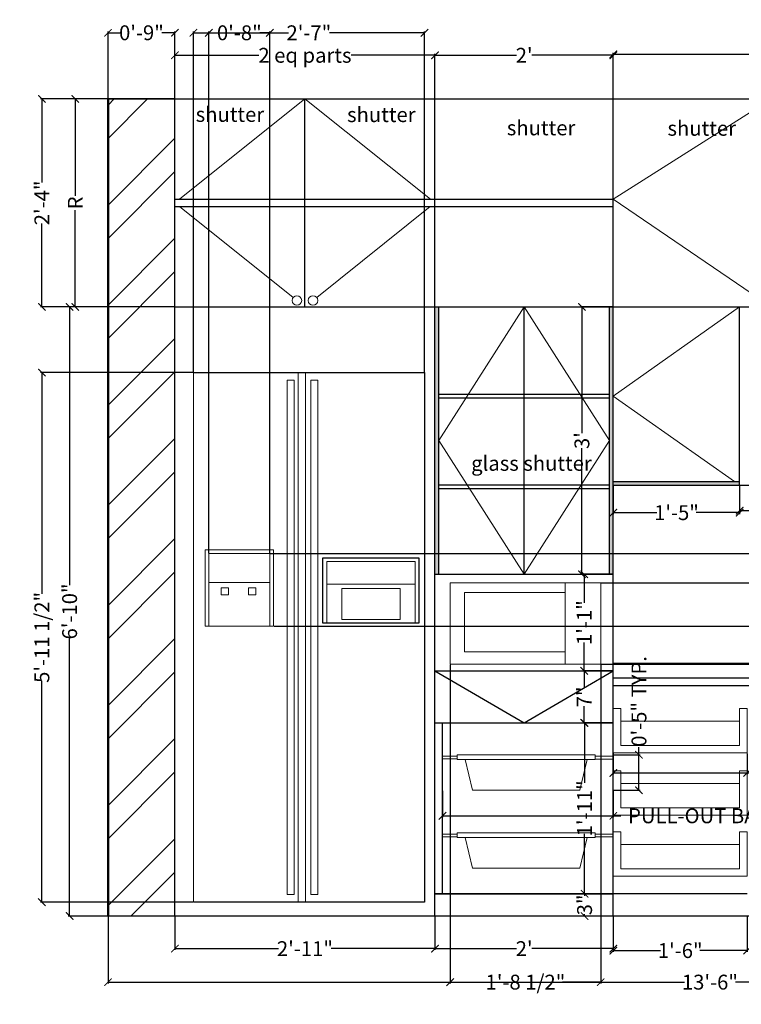
# Model space of a CAD drawing. Units: inches. Extents: x 3107 to 3291, y 1339 to 1621.
# Tile 2 of 3: x 3107 to 3204, y 1489 to 1621. Entities that reach past the tile are written whole.
import ezdxf

# ---------------------------------------------------------------- set-up
doc = ezdxf.new("R2010")
doc.units = ezdxf.units.IN
for name, color, linetype, lineweight in [('A-ANNO-DIMS', 2, 'Continuous', 18), ('A-ANNO-TEXT', 7, 'Continuous', 18), ('A-ELEV', 7, 'Continuous', 25), ('A-ELEV-OPEN', 165, 'Continuous', 13), ('A-ELEV-PATT', 8, 'Continuous', 13), ('A-EQPM', 3, 'Continuous', 18), ('A-FURN', 5, 'Continuous', 18), ('A-WALL', 7, 'Continuous', 50), ('A-WALL-PATT', 8, 'Continuous', 13)]:
    doc.layers.add(name, color=color, linetype=linetype, lineweight=lineweight)
doc.styles.get("Standard").update_dxf_attribs({"font": 'arial.ttf', "height": 2})
doc.dimstyles.get("Standard").update_dxf_attribs({"dimtxt": 2, "dimasz": 1, "dimexe": 0.18, "dimexo": 0.0625, "dimgap": 0.09, "dimtad": 0, "dimdec": 0, "dimzin": 0, "dimdsep": 46, "dimlunit": 3, "dimtxsty": 'Standard', "dimblk": 'ARCHTICK', "dimcen": 0.09, "dimadec": 0, "dimazin": 0, "dimtfac": 1, "dimtdec": 0, "dimtofl": 0, "dimtmove": 0, "dimatfit": 3, "dimfxl": 1, "dimtolj": 1, "dimtzin": 0, "dimarcsym": 0})

# ---------------------------------------------------------------- blocks, each defined once
blk = doc.blocks.new('_ArchTick')
at = {"color": 0, "linetype": 'ByBlock', "const_width": 0.15}
blk.add_lwpolyline([(-0.5, -0.5), (0.5, 0.5)], dxfattribs=at)
blk = doc.blocks.new('*D22')
at = {"layer": 'A-ANNO-DIMS', "color": 0, "lineweight": -2, "transparency": 16777216}
for p, q in [((3203.52, 1558.6), (3203.52, 1555.06)), ((3235.52, 1558.6), (3235.52, 1555.06)), ((3203.52, 1555.24), (3216.75, 1555.24)), ((3235.52, 1555.24), (3222.28, 1555.24))]:
    blk.add_line(p, q, dxfattribs=at)
at = {"layer": 'Defpoints', "color": 0, "transparency": 16777216}
for p in [(3203.52, 1558.66), (3235.52, 1558.66), (3203.52, 1555.24)]:
    blk.add_point(p, dxfattribs=at)
at = {"layer": 'A-ANNO-DIMS', "color": 0, "lineweight": -2, "transparency": 16777216, "rotation": 180}
blk.add_blockref('_ArchTick', (3203.52, 1555.24), dxfattribs=at)
at = {"layer": 'A-ANNO-DIMS', "color": 0, "lineweight": -2, "transparency": 16777216}
blk.add_blockref('_ArchTick', (3235.52, 1555.24), dxfattribs=at)
at = {"layer": 'A-ANNO-DIMS', "color": 0, "transparency": 16777216, "insert": (3219.52, 1555.24), "char_height": 2, "attachment_point": 5}
blk.add_mtext('\\A1;2\'-8"', dxfattribs=at)
blk = doc.blocks.new('*D23')
at = {"layer": 'A-ANNO-DIMS', "color": 0, "lineweight": -2, "transparency": 16777216}
for p, q in [((3186.52, 1558.6), (3186.52, 1554.78)), ((3203.52, 1558.6), (3203.52, 1554.78)), ((3186.52, 1554.96), (3192.36, 1554.96)), ((3203.52, 1554.96), (3197.67, 1554.96))]:
    blk.add_line(p, q, dxfattribs=at)
at = {"layer": 'Defpoints', "color": 0, "transparency": 16777216}
for p in [(3186.52, 1558.66), (3203.52, 1558.66), (3186.52, 1554.96)]:
    blk.add_point(p, dxfattribs=at)
at = {"layer": 'A-ANNO-DIMS', "color": 0, "lineweight": -2, "transparency": 16777216, "rotation": 180}
blk.add_blockref('_ArchTick', (3186.52, 1554.96), dxfattribs=at)
at = {"layer": 'A-ANNO-DIMS', "color": 0, "lineweight": -2, "transparency": 16777216}
blk.add_blockref('_ArchTick', (3203.52, 1554.96), dxfattribs=at)
at = {"layer": 'A-ANNO-DIMS', "color": 0, "transparency": 16777216, "insert": (3195.02, 1554.96), "char_height": 2, "attachment_point": 5}
blk.add_mtext('\\A1;1\'-5"', dxfattribs=at)
blk = doc.blocks.new('*D27')
at = {"layer": 'A-ANNO-DIMS', "color": 0, "lineweight": -2, "transparency": 16777216}
for p, q in [((3186.52, 1500.6), (3186.52, 1495.83)), ((3204.52, 1500.6), (3204.52, 1495.83)), ((3186.52, 1496.01), (3192.86, 1496.01)), ((3204.52, 1496.01), (3198.17, 1496.01))]:
    blk.add_line(p, q, dxfattribs=at)
at = {"layer": 'Defpoints', "color": 0, "transparency": 16777216}
for p in [(3186.52, 1500.66), (3204.52, 1500.66), (3186.52, 1496.01)]:
    blk.add_point(p, dxfattribs=at)
at = {"layer": 'A-ANNO-DIMS', "color": 0, "lineweight": -2, "transparency": 16777216, "rotation": 180}
blk.add_blockref('_ArchTick', (3186.52, 1496.01), dxfattribs=at)
at = {"layer": 'A-ANNO-DIMS', "color": 0, "lineweight": -2, "transparency": 16777216}
blk.add_blockref('_ArchTick', (3204.52, 1496.01), dxfattribs=at)
at = {"layer": 'A-ANNO-DIMS', "color": 0, "transparency": 16777216, "insert": (3195.52, 1496.01), "char_height": 2, "attachment_point": 5}
blk.add_mtext('\\A1;1\'-6"', dxfattribs=at)
blk = doc.blocks.new('*D28')
at = {"layer": 'A-ANNO-DIMS', "color": 0, "lineweight": -2, "transparency": 16777216}
for p, q in [((3162.52, 1500.6), (3162.52, 1496.09)), ((3186.52, 1500.6), (3186.52, 1496.09)), ((3162.52, 1496.27), (3173.49, 1496.27)), ((3186.52, 1496.27), (3175.54, 1496.27))]:
    blk.add_line(p, q, dxfattribs=at)
at = {"layer": 'Defpoints', "color": 0, "transparency": 16777216}
for p in [(3162.52, 1500.66), (3186.52, 1500.66), (3162.52, 1496.27)]:
    blk.add_point(p, dxfattribs=at)
at = {"layer": 'A-ANNO-DIMS', "color": 0, "lineweight": -2, "transparency": 16777216, "rotation": 180}
blk.add_blockref('_ArchTick', (3162.52, 1496.27), dxfattribs=at)
at = {"layer": 'A-ANNO-DIMS', "color": 0, "lineweight": -2, "transparency": 16777216}
blk.add_blockref('_ArchTick', (3186.52, 1496.27), dxfattribs=at)
at = {"layer": 'A-ANNO-DIMS', "color": 0, "transparency": 16777216, "insert": (3174.52, 1496.27), "char_height": 2, "attachment_point": 5}
blk.add_mtext("\\A1;2'", dxfattribs=at)
blk = doc.blocks.new('*D29')
at = {"layer": 'A-ANNO-DIMS', "color": 0, "lineweight": -2, "transparency": 16777216}
for p, q in [((3127.52, 1500.6), (3127.52, 1496.09)), ((3162.52, 1500.6), (3162.52, 1496.09)), ((3127.52, 1496.27), (3141.48, 1496.27)), ((3162.52, 1496.27), (3148.56, 1496.27))]:
    blk.add_line(p, q, dxfattribs=at)
at = {"layer": 'Defpoints', "color": 0, "transparency": 16777216}
for p in [(3127.52, 1500.66), (3162.52, 1500.66), (3127.52, 1496.27)]:
    blk.add_point(p, dxfattribs=at)
at = {"layer": 'A-ANNO-DIMS', "color": 0, "lineweight": -2, "transparency": 16777216, "rotation": 180}
blk.add_blockref('_ArchTick', (3127.52, 1496.27), dxfattribs=at)
at = {"layer": 'A-ANNO-DIMS', "color": 0, "lineweight": -2, "transparency": 16777216}
blk.add_blockref('_ArchTick', (3162.52, 1496.27), dxfattribs=at)
at = {"layer": 'A-ANNO-DIMS', "color": 0, "transparency": 16777216, "insert": (3145.02, 1496.27), "char_height": 2, "attachment_point": 5}
blk.add_mtext('\\A1;2\'-11"', dxfattribs=at)
blk = doc.blocks.new('*D34')
at = {"layer": 'A-ANNO-DIMS', "color": 0, "lineweight": -2, "transparency": 16777216}
for p, q in [((3186.52, 1610.72), (3186.52, 1616.85)), ((3186.52, 1616.67), (3222.79, 1616.67)), ((3271.52, 1616.67), (3235.25, 1616.67)), ((3271.52, 1610.72), (3271.52, 1616.85))]:
    blk.add_line(p, q, dxfattribs=at)
at = {"layer": 'Defpoints', "color": 0, "transparency": 16777216}
for p in [(3186.52, 1616.67), (3186.52, 1610.66), (3271.52, 1610.66)]:
    blk.add_point(p, dxfattribs=at)
at = {"layer": 'A-ANNO-DIMS', "color": 0, "lineweight": -2, "transparency": 16777216, "rotation": 180}
blk.add_blockref('_ArchTick', (3186.52, 1616.67), dxfattribs=at)
at = {"layer": 'A-ANNO-DIMS', "color": 0, "lineweight": -2, "transparency": 16777216}
blk.add_blockref('_ArchTick', (3271.52, 1616.67), dxfattribs=at)
at = {"layer": 'A-ANNO-DIMS', "color": 0, "transparency": 16777216, "insert": (3229.02, 1616.67), "char_height": 2, "attachment_point": 5}
blk.add_mtext('\\A1;4 eq parts', dxfattribs=at)
blk = doc.blocks.new('*D35')
at = {"layer": 'A-ANNO-DIMS', "color": 0, "lineweight": -2, "transparency": 16777216}
for p, q in [((3162.52, 1610.72), (3162.52, 1616.71)), ((3162.52, 1616.53), (3173.49, 1616.53)), ((3186.52, 1616.53), (3175.54, 1616.53)), ((3186.52, 1610.72), (3186.52, 1616.71))]:
    blk.add_line(p, q, dxfattribs=at)
at = {"layer": 'Defpoints', "color": 0, "transparency": 16777216}
for p in [(3162.52, 1616.53), (3162.52, 1610.66), (3186.52, 1610.66)]:
    blk.add_point(p, dxfattribs=at)
at = {"layer": 'A-ANNO-DIMS', "color": 0, "lineweight": -2, "transparency": 16777216, "rotation": 180}
blk.add_blockref('_ArchTick', (3162.52, 1616.53), dxfattribs=at)
at = {"layer": 'A-ANNO-DIMS', "color": 0, "lineweight": -2, "transparency": 16777216}
blk.add_blockref('_ArchTick', (3186.52, 1616.53), dxfattribs=at)
at = {"layer": 'A-ANNO-DIMS', "color": 0, "transparency": 16777216, "insert": (3174.52, 1616.53), "char_height": 2, "attachment_point": 5}
blk.add_mtext("\\A1;2'", dxfattribs=at)
blk = doc.blocks.new('*D36')
at = {"layer": 'A-ANNO-DIMS', "color": 0, "lineweight": -2, "transparency": 16777216}
for p, q in [((3127.52, 1610.72), (3127.52, 1616.71)), ((3127.52, 1616.53), (3138.81, 1616.53)), ((3162.52, 1616.53), (3151.23, 1616.53)), ((3162.52, 1610.72), (3162.52, 1616.71))]:
    blk.add_line(p, q, dxfattribs=at)
at = {"layer": 'Defpoints', "color": 0, "transparency": 16777216}
for p in [(3127.52, 1616.53), (3127.52, 1610.66), (3162.52, 1610.66)]:
    blk.add_point(p, dxfattribs=at)
at = {"layer": 'A-ANNO-DIMS', "color": 0, "lineweight": -2, "transparency": 16777216, "rotation": 180}
blk.add_blockref('_ArchTick', (3127.52, 1616.53), dxfattribs=at)
at = {"layer": 'A-ANNO-DIMS', "color": 0, "lineweight": -2, "transparency": 16777216}
blk.add_blockref('_ArchTick', (3162.52, 1616.53), dxfattribs=at)
at = {"layer": 'A-ANNO-DIMS', "color": 0, "transparency": 16777216, "insert": (3145.02, 1616.53), "char_height": 2, "attachment_point": 5}
blk.add_mtext('\\A1;2 eq parts', dxfattribs=at)
blk = doc.blocks.new('*D37')
at = {"layer": 'A-ANNO-DIMS', "color": 0, "lineweight": -2, "transparency": 16777216}
for p, q in [((3127.46, 1610.66), (3113.94, 1610.66)), ((3114.12, 1610.66), (3114.12, 1597.63)), ((3114.12, 1582.66), (3114.12, 1595.69)), ((3127.46, 1582.66), (3113.94, 1582.66))]:
    blk.add_line(p, q, dxfattribs=at)
at = {"layer": 'Defpoints', "color": 0, "transparency": 16777216}
for p in [(3114.12, 1610.66), (3127.52, 1610.66), (3127.52, 1582.66)]:
    blk.add_point(p, dxfattribs=at)
at = {"layer": 'A-ANNO-DIMS', "color": 0, "lineweight": -2, "transparency": 16777216}
for p, rotation in [((3114.12, 1610.66), 90), ((3114.12, 1582.66), 270)]:
    blk.add_blockref('_ArchTick', p, dxfattribs=dict(at, rotation=rotation))
at = {"layer": 'A-ANNO-DIMS', "color": 0, "transparency": 16777216, "insert": (3114.12, 1596.66), "char_height": 2, "attachment_point": 5, "rotation": 90}
blk.add_mtext('\\A1;R ', dxfattribs=at)
blk = doc.blocks.new('*D38')
at = {"layer": 'A-ANNO-DIMS', "color": 0, "lineweight": -2, "transparency": 16777216}
for p, q in [((3118.46, 1582.66), (3113.17, 1582.66)), ((3113.35, 1582.66), (3113.35, 1545.19)), ((3113.35, 1500.66), (3113.35, 1538.13)), ((3118.46, 1500.66), (3113.17, 1500.66))]:
    blk.add_line(p, q, dxfattribs=at)
at = {"layer": 'Defpoints', "color": 0, "transparency": 16777216}
for p in [(3118.52, 1582.66), (3113.35, 1500.66), (3118.52, 1500.66)]:
    blk.add_point(p, dxfattribs=at)
at = {"layer": 'A-ANNO-DIMS', "color": 0, "lineweight": -2, "transparency": 16777216}
for p, rotation in [((3113.35, 1582.66), 90), ((3113.35, 1500.66), 270)]:
    blk.add_blockref('_ArchTick', p, dxfattribs=dict(at, rotation=rotation))
at = {"layer": 'A-ANNO-DIMS', "color": 0, "transparency": 16777216, "insert": (3113.35, 1541.66), "char_height": 2, "attachment_point": 5, "rotation": 90}
blk.add_mtext('\\A1;6\'-10"', dxfattribs=at)
blk = doc.blocks.new('*D40')
at = {"layer": 'A-ANNO-DIMS', "color": 0, "lineweight": -2, "transparency": 16777216}
for p, q in [((3186.46, 1526.66), (3182.47, 1526.66)), ((3182.65, 1526.66), (3182.65, 1518.59)), ((3182.65, 1503.66), (3182.65, 1511.73)), ((3186.46, 1503.66), (3182.47, 1503.66))]:
    blk.add_line(p, q, dxfattribs=at)
at = {"layer": 'Defpoints', "color": 0, "transparency": 16777216}
for p in [(3182.65, 1526.66), (3186.52, 1526.66), (3186.52, 1503.66)]:
    blk.add_point(p, dxfattribs=at)
at = {"layer": 'A-ANNO-DIMS', "color": 0, "lineweight": -2, "transparency": 16777216}
for p, rotation in [((3182.65, 1526.66), 90), ((3182.65, 1503.66), 270)]:
    blk.add_blockref('_ArchTick', p, dxfattribs=dict(at, rotation=rotation))
at = {"layer": 'A-ANNO-DIMS', "color": 0, "transparency": 16777216, "insert": (3182.65, 1515.16), "char_height": 2, "attachment_point": 5, "rotation": 90}
blk.add_mtext('\\A1;1\'-11"', dxfattribs=at)
blk = doc.blocks.new('*D41')
at = {"layer": 'A-ANNO-DIMS', "color": 0, "lineweight": -2, "transparency": 16777216}
for p, q in [((3186.46, 1503.66), (3182.47, 1503.66)), ((3182.65, 1503.66), (3182.65, 1503.4)), ((3186.46, 1500.66), (3182.47, 1500.66)), ((3182.65, 1500.66), (3182.65, 1500.92))]:
    blk.add_line(p, q, dxfattribs=at)
at = {"layer": 'Defpoints', "color": 0, "transparency": 16777216}
for p in [(3182.65, 1503.66), (3186.52, 1503.66), (3186.52, 1500.66)]:
    blk.add_point(p, dxfattribs=at)
at = {"layer": 'A-ANNO-DIMS', "color": 0, "lineweight": -2, "transparency": 16777216}
for p, rotation in [((3182.65, 1503.66), 90), ((3182.65, 1500.66), 270)]:
    blk.add_blockref('_ArchTick', p, dxfattribs=dict(at, rotation=rotation))
at = {"layer": 'A-ANNO-DIMS', "color": 0, "transparency": 16777216, "insert": (3182.65, 1502.16), "char_height": 2, "attachment_point": 5, "rotation": 90}
blk.add_mtext('\\A1;3"', dxfattribs=at)
blk = doc.blocks.new('*D42')
at = {"layer": 'A-ANNO-DIMS', "color": 0, "lineweight": -2, "transparency": 16777216}
for p, q in [((3186.46, 1533.66), (3182.42, 1533.66)), ((3182.6, 1533.66), (3182.6, 1531.39)), ((3182.6, 1526.66), (3182.6, 1528.93)), ((3186.46, 1526.66), (3182.42, 1526.66))]:
    blk.add_line(p, q, dxfattribs=at)
at = {"layer": 'Defpoints', "color": 0, "transparency": 16777216}
for p in [(3182.6, 1533.66), (3186.52, 1533.66), (3186.52, 1526.66)]:
    blk.add_point(p, dxfattribs=at)
at = {"layer": 'A-ANNO-DIMS', "color": 0, "lineweight": -2, "transparency": 16777216}
for p, rotation in [((3182.6, 1533.66), 90), ((3182.6, 1526.66), 270)]:
    blk.add_blockref('_ArchTick', p, dxfattribs=dict(at, rotation=rotation))
at = {"layer": 'A-ANNO-DIMS', "color": 0, "transparency": 16777216, "insert": (3182.6, 1530.16), "char_height": 2, "attachment_point": 5, "rotation": 90}
blk.add_mtext('\\A1;7"', dxfattribs=at)
blk = doc.blocks.new('*D43')
at = {"layer": 'A-ANNO-DIMS', "color": 0, "lineweight": -2, "transparency": 16777216}
for p, q in [((3186.46, 1546.66), (3182.42, 1546.66)), ((3182.6, 1546.66), (3182.6, 1542.81)), ((3182.6, 1533.66), (3182.6, 1537.5)), ((3186.46, 1533.66), (3182.42, 1533.66))]:
    blk.add_line(p, q, dxfattribs=at)
at = {"layer": 'Defpoints', "color": 0, "transparency": 16777216}
for p in [(3182.6, 1546.66), (3186.52, 1546.66), (3186.52, 1533.66)]:
    blk.add_point(p, dxfattribs=at)
at = {"layer": 'A-ANNO-DIMS', "color": 0, "lineweight": -2, "transparency": 16777216}
for p, rotation in [((3182.6, 1546.66), 90), ((3182.6, 1533.66), 270)]:
    blk.add_blockref('_ArchTick', p, dxfattribs=dict(at, rotation=rotation))
at = {"layer": 'A-ANNO-DIMS', "color": 0, "transparency": 16777216, "insert": (3182.6, 1540.16), "char_height": 2, "attachment_point": 5, "rotation": 90}
blk.add_mtext('\\A1;1\'-1"', dxfattribs=at)
blk = doc.blocks.new('*D44')
at = {"layer": 'A-ANNO-DIMS', "color": 0, "lineweight": -2, "transparency": 16777216}
for p, q in [((3186.46, 1582.66), (3182.11, 1582.66)), ((3182.29, 1582.66), (3182.29, 1565.67)), ((3182.29, 1546.66), (3182.29, 1563.65)), ((3186.46, 1546.66), (3182.11, 1546.66))]:
    blk.add_line(p, q, dxfattribs=at)
at = {"layer": 'Defpoints', "color": 0, "transparency": 16777216}
for p in [(3182.29, 1582.66), (3186.52, 1582.66), (3186.52, 1546.66)]:
    blk.add_point(p, dxfattribs=at)
at = {"layer": 'A-ANNO-DIMS', "color": 0, "lineweight": -2, "transparency": 16777216}
for p, rotation in [((3182.29, 1582.66), 90), ((3182.29, 1546.66), 270)]:
    blk.add_blockref('_ArchTick', p, dxfattribs=dict(at, rotation=rotation))
at = {"layer": 'A-ANNO-DIMS', "color": 0, "transparency": 16777216, "insert": (3182.29, 1564.66), "char_height": 2, "attachment_point": 5, "rotation": 90}
blk.add_mtext("\\A1;3'", dxfattribs=at)
blk = doc.blocks.new('DRAWER-TRAY')
for p, q in [((3186.52, 1528.59), (3187.52, 1528.59)), ((3186.52, 1522.62), (3186.52, 1528.59)), ((3187.52, 1523.62), (3187.52, 1528.59)), ((3203.52, 1528.59), (3203.52, 1523.62)), ((3203.52, 1528.59), (3204.52, 1528.59)), ((3204.52, 1528.59), (3204.52, 1522.62)), ((3187.52, 1526.9), (3203.52, 1526.9)), ((3203.52, 1523.62), (3187.52, 1523.62)), ((3204.52, 1522.62), (3186.52, 1522.62))]:
    blk.add_line(p, q)
blk = doc.blocks.new('PULLOUT-BASKET')
for p, q in [((3163.52, 1522.18), (3165.49, 1522.18)), ((3165.49, 1521.83), (3163.52, 1521.83)), ((3166.58, 1521.72), (3167.55, 1517.6)), ((3182.98, 1521.72), (3182.01, 1517.6)), ((3184.07, 1522.16), (3186.52, 1522.16)), ((3184.07, 1521.79), (3186.52, 1521.79)), ((3167.55, 1517.6), (3182.01, 1517.6))]:
    blk.add_line(p, q)
blk.add_lwpolyline([(3165.49, 1522.37), (3184.07, 1522.37), (3184.07, 1521.72), (3165.49, 1521.72)], close=True)
blk = doc.blocks.new('*D50')
at = {"layer": 'A-ANNO-DIMS', "color": 0, "lineweight": -2, "transparency": 16777216}
for p, q in [((3186.52, 1522.56), (3186.52, 1519.74)), ((3204.52, 1522.56), (3204.52, 1519.74)), ((3186.52, 1519.92), (3204.52, 1519.92)), ((3204.52, 1519.92), (3205.52, 1519.92))]:
    blk.add_line(p, q, dxfattribs=at)
at = {"layer": 'Defpoints', "color": 0, "transparency": 16777216}
for p in [(3186.52, 1522.62), (3204.52, 1522.62), (3204.52, 1519.92)]:
    blk.add_point(p, dxfattribs=at)
at = {"layer": 'A-ANNO-DIMS', "color": 0, "lineweight": -2, "transparency": 16777216, "rotation": 180}
blk.add_blockref('_ArchTick', (3186.52, 1519.92), dxfattribs=at)
at = {"layer": 'A-ANNO-DIMS', "color": 0, "lineweight": -2, "transparency": 16777216}
blk.add_blockref('_ArchTick', (3204.52, 1519.92), dxfattribs=at)
at = {"layer": 'A-ANNO-DIMS', "color": 0, "transparency": 16777216, "insert": (3222.36, 1519.92), "char_height": 2, "attachment_point": 5}
blk.add_mtext('\\A1;DRAWER TRAY 1\'-6" TYP.', dxfattribs=at)
blk = doc.blocks.new('*D52')
at = {"layer": 'A-ANNO-DIMS', "color": 0, "lineweight": -2, "transparency": 16777216}
for p, q in [((3163.52, 1517.53), (3163.52, 1513.97)), ((3186.52, 1517.53), (3186.52, 1513.97)), ((3163.52, 1514.15), (3186.52, 1514.15)), ((3186.52, 1514.15), (3187.52, 1514.15))]:
    blk.add_line(p, q, dxfattribs=at)
at = {"layer": 'Defpoints', "color": 0, "transparency": 16777216}
for p in [(3163.52, 1517.6), (3186.52, 1517.6), (3186.52, 1514.15)]:
    blk.add_point(p, dxfattribs=at)
at = {"layer": 'A-ANNO-DIMS', "color": 0, "lineweight": -2, "transparency": 16777216, "rotation": 180}
blk.add_blockref('_ArchTick', (3163.52, 1514.15), dxfattribs=at)
at = {"layer": 'A-ANNO-DIMS', "color": 0, "lineweight": -2, "transparency": 16777216}
blk.add_blockref('_ArchTick', (3186.52, 1514.15), dxfattribs=at)
at = {"layer": 'A-ANNO-DIMS', "color": 0, "transparency": 16777216, "insert": (3207.63, 1514.15), "char_height": 2, "attachment_point": 5}
blk.add_mtext('\\A1;PULL-OUT BASKET 1\'-11" TYP.', dxfattribs=at)
blk = doc.blocks.new('*D53')
at = {"layer": 'A-ANNO-DIMS', "color": 0, "lineweight": -2, "transparency": 16777216}
for p, q in [((3189.97, 1522.37), (3189.97, 1523.37)), ((3186.58, 1522.37), (3190.15, 1522.37)), ((3189.97, 1517.6), (3189.97, 1522.37)), ((3186.58, 1517.6), (3190.15, 1517.6))]:
    blk.add_line(p, q, dxfattribs=at)
at = {"layer": 'Defpoints', "color": 0, "transparency": 16777216}
for p in [(3186.52, 1522.37), (3189.97, 1522.37), (3186.52, 1517.6)]:
    blk.add_point(p, dxfattribs=at)
at = {"layer": 'A-ANNO-DIMS', "color": 0, "lineweight": -2, "transparency": 16777216}
for p, rotation in [((3189.97, 1522.37), 90), ((3189.97, 1517.6), 270)]:
    blk.add_blockref('_ArchTick', p, dxfattribs=dict(at, rotation=rotation))
at = {"layer": 'A-ANNO-DIMS', "color": 0, "transparency": 16777216, "insert": (3189.97, 1529.55), "char_height": 2, "attachment_point": 5, "rotation": 90}
blk.add_mtext('\\A1;0\'-5" TYP.', dxfattribs=at)
blk = doc.blocks.new('*D54')
at = {"layer": 'A-ANNO-DIMS', "color": 0, "lineweight": -2, "transparency": 16777216}
for p, q in [((3130.01, 1573.89), (3130.01, 1619.74)), ((3161.1, 1573.89), (3161.1, 1619.74)), ((3130.01, 1619.56), (3142.79, 1619.56)), ((3161.1, 1619.56), (3148.32, 1619.56))]:
    blk.add_line(p, q, dxfattribs=at)
at = {"layer": 'Defpoints', "color": 0, "transparency": 16777216}
for p in [(3161.1, 1619.56), (3130.01, 1573.82), (3161.1, 1573.82)]:
    blk.add_point(p, dxfattribs=at)
at = {"layer": 'A-ANNO-DIMS', "color": 0, "lineweight": -2, "transparency": 16777216, "rotation": 180}
blk.add_blockref('_ArchTick', (3130.01, 1619.56), dxfattribs=at)
at = {"layer": 'A-ANNO-DIMS', "color": 0, "lineweight": -2, "transparency": 16777216}
blk.add_blockref('_ArchTick', (3161.1, 1619.56), dxfattribs=at)
at = {"layer": 'A-ANNO-DIMS', "color": 0, "transparency": 16777216, "insert": (3145.55, 1619.56), "char_height": 2, "attachment_point": 5}
blk.add_mtext('\\A1;2\'-7"', dxfattribs=at)
blk = doc.blocks.new('*D55')
at = {"layer": 'A-ANNO-DIMS', "color": 0, "lineweight": -2, "transparency": 16777216}
for p, q in [((3164.56, 1534.48), (3164.56, 1491.58)), ((3184.82, 1534.48), (3184.82, 1491.58)), ((3164.56, 1491.76), (3169.71, 1491.76)), ((3184.82, 1491.76), (3179.67, 1491.76))]:
    blk.add_line(p, q, dxfattribs=at)
at = {"layer": 'Defpoints', "color": 0, "transparency": 16777216}
for p in [(3164.56, 1534.55), (3184.82, 1534.55), (3184.82, 1491.76)]:
    blk.add_point(p, dxfattribs=at)
at = {"layer": 'A-ANNO-DIMS', "color": 0, "lineweight": -2, "transparency": 16777216, "rotation": 180}
blk.add_blockref('_ArchTick', (3164.56, 1491.76), dxfattribs=at)
at = {"layer": 'A-ANNO-DIMS', "color": 0, "lineweight": -2, "transparency": 16777216}
blk.add_blockref('_ArchTick', (3184.82, 1491.76), dxfattribs=at)
at = {"layer": 'A-ANNO-DIMS', "color": 0, "transparency": 16777216, "insert": (3174.69, 1491.76), "char_height": 2, "attachment_point": 5}
blk.add_mtext('\\A1;1\'-8 1/2"', dxfattribs=at)
blk = doc.blocks.new('*D57')
at = {"layer": 'A-ANNO-DIMS', "color": 0, "lineweight": -2, "transparency": 16777216}
for p, q in [((3118.46, 1610.66), (3109.44, 1610.66)), ((3109.62, 1610.66), (3109.62, 1599.42)), ((3109.62, 1582.66), (3109.62, 1593.89)), ((3118.46, 1582.66), (3109.44, 1582.66))]:
    blk.add_line(p, q, dxfattribs=at)
at = {"layer": 'Defpoints', "color": 0, "transparency": 16777216}
for p in [(3109.62, 1610.66), (3118.52, 1610.66), (3118.52, 1582.66)]:
    blk.add_point(p, dxfattribs=at)
at = {"layer": 'A-ANNO-DIMS', "color": 0, "lineweight": -2, "transparency": 16777216}
for p, rotation in [((3109.62, 1610.66), 90), ((3109.62, 1582.66), 270)]:
    blk.add_blockref('_ArchTick', p, dxfattribs=dict(at, rotation=rotation))
at = {"layer": 'A-ANNO-DIMS', "color": 0, "transparency": 16777216, "insert": (3109.62, 1596.66), "char_height": 2, "attachment_point": 5, "rotation": 90}
blk.add_mtext('\\A1;2\'-4"', dxfattribs=at)
blk = doc.blocks.new('*D58')
at = {"layer": 'A-ANNO-DIMS', "color": 0, "lineweight": -2, "transparency": 16777216}
for p, q in [((3118.52, 1610.72), (3118.52, 1619.74)), ((3127.52, 1610.72), (3127.52, 1619.74)), ((3118.52, 1619.56), (3120.27, 1619.56)), ((3127.52, 1619.56), (3125.77, 1619.56))]:
    blk.add_line(p, q, dxfattribs=at)
at = {"layer": 'Defpoints', "color": 0, "transparency": 16777216}
for p in [(3127.52, 1619.56), (3118.52, 1610.66), (3127.52, 1610.66)]:
    blk.add_point(p, dxfattribs=at)
at = {"layer": 'A-ANNO-DIMS', "color": 0, "lineweight": -2, "transparency": 16777216, "rotation": 180}
blk.add_blockref('_ArchTick', (3118.52, 1619.56), dxfattribs=at)
at = {"layer": 'A-ANNO-DIMS', "color": 0, "lineweight": -2, "transparency": 16777216}
blk.add_blockref('_ArchTick', (3127.52, 1619.56), dxfattribs=at)
at = {"layer": 'A-ANNO-DIMS', "color": 0, "transparency": 16777216, "insert": (3123.02, 1619.56), "char_height": 2, "attachment_point": 5}
blk.add_mtext('\\A1;0\'-9"', dxfattribs=at)
blk = doc.blocks.new('*D60')
at = {"layer": 'A-ANNO-DIMS', "color": 0, "lineweight": -2, "transparency": 16777216}
for p, q in [((3129.95, 1573.82), (3109.44, 1573.82)), ((3109.62, 1573.82), (3109.62, 1544.03)), ((3109.62, 1502.52), (3109.62, 1532.32)), ((3129.95, 1502.52), (3109.44, 1502.52))]:
    blk.add_line(p, q, dxfattribs=at)
at = {"layer": 'Defpoints', "color": 0, "transparency": 16777216}
for p in [(3109.62, 1573.82), (3130.01, 1573.82), (3130.01, 1502.52)]:
    blk.add_point(p, dxfattribs=at)
at = {"layer": 'A-ANNO-DIMS', "color": 0, "lineweight": -2, "transparency": 16777216}
for p, rotation in [((3109.62, 1573.82), 90), ((3109.62, 1502.52), 270)]:
    blk.add_blockref('_ArchTick', p, dxfattribs=dict(at, rotation=rotation))
at = {"layer": 'A-ANNO-DIMS', "color": 0, "transparency": 16777216, "insert": (3109.62, 1538.17), "char_height": 2, "attachment_point": 5, "rotation": 90}
blk.add_mtext('\\A1;5\'-11 1/2"', dxfattribs=at)
blk = doc.blocks.new('*D61')
at = {"layer": 'A-ANNO-DIMS', "color": 0, "lineweight": -2, "transparency": 16777216}
for p, q in [((3132.08, 1549.52), (3132.08, 1619.74)), ((3140.3, 1549.52), (3140.3, 1619.74)), ((3132.08, 1619.56), (3133.44, 1619.56)), ((3140.3, 1619.56), (3138.94, 1619.56))]:
    blk.add_line(p, q, dxfattribs=at)
at = {"layer": 'Defpoints', "color": 0, "transparency": 16777216}
for p in [(3140.3, 1619.56), (3132.08, 1549.46), (3140.3, 1549.46)]:
    blk.add_point(p, dxfattribs=at)
at = {"layer": 'A-ANNO-DIMS', "color": 0, "lineweight": -2, "transparency": 16777216, "rotation": 180}
blk.add_blockref('_ArchTick', (3132.08, 1619.56), dxfattribs=at)
at = {"layer": 'A-ANNO-DIMS', "color": 0, "lineweight": -2, "transparency": 16777216}
blk.add_blockref('_ArchTick', (3140.3, 1619.56), dxfattribs=at)
at = {"layer": 'A-ANNO-DIMS', "color": 0, "transparency": 16777216, "insert": (3136.19, 1619.56), "char_height": 2, "attachment_point": 5}
blk.add_mtext('\\A1;0\'-8"', dxfattribs=at)
blk = doc.blocks.new('*D62')
at = {"layer": 'A-ANNO-DIMS', "color": 0, "lineweight": -2, "transparency": 16777216}
for p, q in [((3140.37, 1549.46), (3289.6, 1549.46)), ((3289.42, 1549.46), (3289.42, 1548.09)), ((3289.42, 1539.66), (3289.42, 1541.04)), ((3140.87, 1539.66), (3289.6, 1539.66))]:
    blk.add_line(p, q, dxfattribs=at)
at = {"layer": 'Defpoints', "color": 0, "transparency": 16777216}
for p in [(3140.3, 1549.46), (3289.42, 1549.46), (3140.8, 1539.66)]:
    blk.add_point(p, dxfattribs=at)
at = {"layer": 'A-ANNO-DIMS', "color": 0, "lineweight": -2, "transparency": 16777216}
for p, rotation in [((3289.42, 1549.46), 90), ((3289.42, 1539.66), 270)]:
    blk.add_blockref('_ArchTick', p, dxfattribs=dict(at, rotation=rotation))
at = {"layer": 'A-ANNO-DIMS', "color": 0, "transparency": 16777216, "insert": (3289.42, 1544.56), "char_height": 2, "attachment_point": 5, "rotation": 90}
blk.add_mtext('\\A1;0\'-10"', dxfattribs=at)
blk = doc.blocks.new('*D63')
at = {"layer": 'A-ANNO-DIMS', "color": 0, "lineweight": -2, "transparency": 16777216}
for p, q in [((3184.88, 1545.5), (3289.6, 1545.5)), ((3289.42, 1545.5), (3289.42, 1543.55)), ((3289.42, 1534.55), (3289.42, 1536.5)), ((3184.88, 1534.55), (3289.6, 1534.55))]:
    blk.add_line(p, q, dxfattribs=at)
at = {"layer": 'Defpoints', "color": 0, "transparency": 16777216}
for p in [(3184.82, 1545.5), (3289.42, 1545.5), (3184.82, 1534.55)]:
    blk.add_point(p, dxfattribs=at)
at = {"layer": 'A-ANNO-DIMS', "color": 0, "lineweight": -2, "transparency": 16777216}
for p, rotation in [((3289.42, 1545.5), 90), ((3289.42, 1534.55), 270)]:
    blk.add_blockref('_ArchTick', p, dxfattribs=dict(at, rotation=rotation))
at = {"layer": 'A-ANNO-DIMS', "color": 0, "transparency": 16777216, "insert": (3289.42, 1540.02), "char_height": 2, "attachment_point": 5, "rotation": 90}
blk.add_mtext('\\A1;0\'-11"', dxfattribs=at)
blk = doc.blocks.new('*D67')
at = {"layer": 'A-ANNO-DIMS', "color": 0, "lineweight": -2, "transparency": 16777216}
for p, q in [((3118.52, 1500.6), (3118.52, 1491.58)), ((3280.52, 1500.6), (3280.52, 1491.58)), ((3118.52, 1491.76), (3196.09, 1491.76)), ((3280.52, 1491.76), (3202.95, 1491.76))]:
    blk.add_line(p, q, dxfattribs=at)
at = {"layer": 'Defpoints', "color": 0, "transparency": 16777216}
for p in [(3118.52, 1500.66), (3280.52, 1500.66), (3280.52, 1491.76)]:
    blk.add_point(p, dxfattribs=at)
at = {"layer": 'A-ANNO-DIMS', "color": 0, "lineweight": -2, "transparency": 16777216, "rotation": 180}
blk.add_blockref('_ArchTick', (3118.52, 1491.76), dxfattribs=at)
at = {"layer": 'A-ANNO-DIMS', "color": 0, "lineweight": -2, "transparency": 16777216}
blk.add_blockref('_ArchTick', (3280.52, 1491.76), dxfattribs=at)
at = {"layer": 'A-ANNO-DIMS', "color": 0, "transparency": 16777216, "insert": (3199.52, 1491.76), "char_height": 2, "attachment_point": 5}
blk.add_mtext('\\A1;13\'-6"', dxfattribs=at)

msp = doc.modelspace()

# ---------------------------------------------------------------- hatches: boundary and pattern name
at = {"layer": 'A-ELEV-PATT'}
h = msp.add_hatch(color=256, dxfattribs=at)
h.dxf.hatch_style = 1
h.paths.add_polyline_path([(3163.02, 1582.66), (3162.52, 1582.66), (3162.52, 1546.66), (3163.02, 1546.66)])
h.paths.add_polyline_path([(3186.52, 1582.66), (3186.02, 1582.66), (3186.02, 1546.66), (3186.52, 1546.66), (3186.52, 1558.66)])
h = msp.add_hatch(color=256, dxfattribs=at)
h.dxf.hatch_style = 1
h.paths.add_polyline_path([(3203.52, 1559.16), (3186.52, 1559.16), (3186.52, 1558.66), (3203.52, 1558.66)])
at = {"layer": 'A-WALL-PATT'}
h = msp.add_hatch(dxfattribs=at)
h.set_pattern_fill('ANSI32', color=256)
h.paths.add_polyline_path([(3280.52, 1582.66), (3280.52, 1610.66), (3271.52, 1610.66), (3271.52, 1534.66), (3271.52, 1500.66), (3280.52, 1500.66)])
h.paths.add_polyline_path([(3127.52, 1582.66), (3118.52, 1582.66), (3118.52, 1500.66), (3127.52, 1500.66)])
h.paths.add_polyline_path([(3127.52, 1610.66), (3118.52, 1610.66), (3118.52, 1582.66), (3127.52, 1582.66)])

# ---------------------------------------------------------------- linework, layer by layer
at = {"layer": 'A-ELEV'}
for p, q in [((3118.52, 1610.66), (3280.52, 1610.66)), ((3127.52, 1500.66), (3127.52, 1610.66)), ((3145.02, 1582.66), (3145.02, 1610.66)), ((3162.52, 1526.66), (3162.52, 1610.66)), ((3186.52, 1582.66), (3186.52, 1610.66)), ((3127.52, 1597.16), (3186.52, 1597.16)), ((3127.52, 1596.16), (3186.52, 1596.16)), ((3127.52, 1582.66), (3271.52, 1582.66)), ((3163.02, 1546.66), (3163.02, 1582.66)), ((3174.52, 1546.66), (3174.52, 1582.66)), ((3186.02, 1546.66), (3186.02, 1582.66)), ((3186.52, 1558.66), (3186.52, 1582.66)), ((3203.52, 1558.66), (3203.52, 1582.66)), ((3130.01, 1573.82), (3161.1, 1573.82)), ((3161.1, 1573.82), (3161.1, 1502.52)), ((3163.02, 1570.91), (3186.02, 1570.91)), ((3163.02, 1570.41), (3186.02, 1570.41)), ((3186.52, 1559.16), (3203.52, 1559.16)), ((3186.52, 1559.16), (3203.52, 1559.16)), ((3186.02, 1558.66), (3163.02, 1558.66)), ((3186.02, 1558.16), (3163.02, 1558.16)), ((3186.52, 1500.66), (3186.52, 1558.66)), ((3186.52, 1558.66), (3271.52, 1558.66)), ((3162.52, 1546.66), (3186.52, 1546.66)), ((3162.52, 1533.66), (3186.52, 1533.66)), ((3162.52, 1533.66), (3174.52, 1526.66)), ((3174.52, 1526.66), (3186.52, 1533.66)), ((3271.52, 1534.66), (3186.52, 1534.66)), ((3247.52, 1532.66), (3186.52, 1532.66)), ((3247.52, 1531.66), (3186.52, 1531.66)), ((3162.52, 1500.66), (3162.52, 1526.66)), ((3162.52, 1526.66), (3186.52, 1526.66)), ((3163.52, 1503.66), (3163.52, 1526.66)), ((3162.52, 1503.66), (3186.52, 1503.66)), ((3204.52, 1503.66), (3162.52, 1503.66)), ((3161.1, 1502.52), (3130.01, 1502.52)), ((3280.52, 1500.66), (3118.52, 1500.66))]:
    msp.add_line(p, q, dxfattribs=at)
msp.add_lwpolyline([(3147.45, 1548.87), (3160.35, 1548.87), (3160.35, 1540.07), (3147.45, 1540.07)], close=True, dxfattribs=at)
at = {"layer": 'A-ELEV-OPEN'}
for p, q in [((3128.12, 1597.16), (3145.02, 1610.66)), ((3161.91, 1597.16), (3145.02, 1610.66)), ((3207.77, 1610.66), (3186.52, 1597.16)), ((3143.44, 1583.92), (3128.16, 1596.16)), ((3146.6, 1583.92), (3161.87, 1596.16)), ((3186.52, 1597.16), (3206.19, 1583.74)), ((3163.02, 1564.66), (3174.52, 1582.66)), ((3186.02, 1564.66), (3174.52, 1582.66)), ((3203.52, 1582.66), (3186.52, 1570.66)), ((3186.52, 1570.66), (3202.81, 1559.16)), ((3174.52, 1546.66), (3163.02, 1564.66)), ((3174.52, 1546.66), (3186.02, 1564.66))]:
    msp.add_line(p, q, dxfattribs=at)
for centre in [(3143.94, 1583.52), (3146.1, 1583.52)]:
    msp.add_circle(centre, 0.642, dxfattribs=at)
at = {"layer": 'A-EQPM'}
for p, q in [((3130.01, 1502.52), (3130.01, 1573.82)), ((3144.1, 1573.82), (3144.1, 1502.52)), ((3145.1, 1573.82), (3145.1, 1502.52)), ((3132.08, 1549.46), (3140.3, 1549.46)), ((3132.08, 1539.66), (3132.08, 1549.46)), ((3140.3, 1549.46), (3140.3, 1539.66)), ((3147.95, 1548.37), (3159.85, 1548.37)), ((3147.95, 1540.07), (3147.95, 1548.37)), ((3159.85, 1548.37), (3159.85, 1540.07)), ((3140.3, 1545.57), (3132.08, 1545.57)), ((3180.05, 1545.5), (3180.05, 1534.55)), ((3147.95, 1545.32), (3159.85, 1545.32)), ((3166.51, 1544.23), (3180.05, 1544.23)), ((3166.51, 1536.21), (3166.51, 1544.23)), ((3180.05, 1536.21), (3166.51, 1536.21))]:
    msp.add_line(p, q, dxfattribs=at)
for points in [[(3142.63, 1572.78), (3143.58, 1572.78), (3143.58, 1503.57), (3142.63, 1503.57)], [(3145.8, 1572.78), (3146.75, 1572.78), (3146.75, 1503.57), (3145.8, 1503.57)], [(3131.58, 1549.96), (3140.8, 1549.96), (3140.8, 1539.66), (3131.58, 1539.66)], [(3164.56, 1545.5), (3184.82, 1545.5), (3184.82, 1534.55), (3164.56, 1534.55)], [(3133.75, 1544.84), (3134.73, 1544.84), (3134.73, 1543.9), (3133.75, 1543.9)], [(3137.41, 1544.84), (3138.39, 1544.84), (3138.39, 1543.9), (3137.41, 1543.9)], [(3150, 1544.75), (3157.82, 1544.75), (3157.82, 1540.59), (3150, 1540.59)]]:
    msp.add_lwpolyline(points, close=True, dxfattribs=at)
at = {"layer": 'A-WALL'}
for p, q in [((3118.52, 1582.66), (3118.52, 1610.66)), ((3118.52, 1500.66), (3118.52, 1582.66))]:
    msp.add_line(p, q, dxfattribs=at)

# ---------------------------------------------------------------- block references
at = {"layer": 'A-FURN'}
for name, p in [('DRAWER-TRAY', (0, 0)), ('PULLOUT-BASKET', (0, 0)), ('DRAWER-TRAY', (0, -8.39)), ('PULLOUT-BASKET', (0, -10.49)), ('DRAWER-TRAY', (0, -16.6))]:
    msp.add_blockref(name, p, dxfattribs=at)

# ---------------------------------------------------------------- texts
at = {"layer": 'A-ANNO-TEXT', "char_height": 2, "attachment_point": 1}
for s, width, insert in [('shutter', 10.538, (3130.32, 1609.57)), ('shutter', 9.0986, (3150.69, 1609.54)), ('shutter ', 10.907, (3172.19, 1607.76)), ('shutter ', 13.0813, (3193.81, 1607.7)), ('glass shutter', 16.5545, (3167.39, 1562.6))]:
    msp.add_mtext_dynamic_manual_height_columns(s, width=width, gutter_width=10, heights=[0], dxfattribs=dict(at, insert=insert))

# ---------------------------------------------------------------- dimensions: what is measured, and where the dimension line sits
at = {"layer": 'A-ANNO-DIMS'}
for base, p1, p2, text, override, picture, middle in [((3127.52, 1616.53), (3162.52, 1610.66), (3127.52, 1610.66), '2 eq parts', {"dimclrd": 0, "dimclre": 0, "dimclrt": 0}, '*D36', (3145.02, 1616.53)), ((3186.52, 1616.67), (3271.52, 1610.66), (3186.52, 1610.66), '4 eq parts', {"dimclrd": 0, "dimclre": 0, "dimclrt": 0}, '*D34', (3229.02, 1616.67)), ((3204.52, 1519.92), (3186.52, 1522.62), (3204.52, 1522.62), 'DRAWER TRAY <> TYP.', {"dimdec": 1, "dimrnd": 0, "dimzin": 1, "dimlunit": 4, "dimfrac": 2}, '*D50', (3222.36, 1519.92)), ((3186.52, 1514.15), (3163.52, 1517.6), (3186.52, 1517.6), 'PULL-OUT BASKET <> TYP.', {"dimdec": 1, "dimrnd": 0, "dimzin": 1, "dimlunit": 4, "dimfrac": 2}, '*D52', (3207.63, 1514.15))]:
    dim = msp.add_linear_dim(base=base, p1=p1, p2=p2, text=text, dimstyle='Standard', override=override, dxfattribs=at)
    dim.commit()
    dim.dimension.update_dxf_attribs({"geometry": picture, "text_midpoint": middle})
for base, p1, p2, override, picture, middle in [((3127.52, 1619.56), (3118.52, 1610.66), (3127.52, 1610.66), {"dimdec": 1, "dimlfac": 1, "dimrnd": 0, "dimzin": 1, "dimdsep": 46, "dimlunit": 4, "dimfrac": 2}, '*D58', (3123.02, 1619.56)), ((3161.1, 1619.56), (3130.01, 1573.82), (3161.1, 1573.82), {"dimdec": 1, "dimlfac": 1, "dimrnd": 0, "dimzin": 1, "dimdsep": 46, "dimlunit": 4, "dimfrac": 2}, '*D54', (3145.55, 1619.56)), ((3140.3, 1619.56), (3132.08, 1549.46), (3140.3, 1549.46), {"dimdec": 1, "dimlfac": 1, "dimrnd": 0, "dimzin": 1, "dimdsep": 46, "dimlunit": 4, "dimfrac": 2}, '*D61', (3136.19, 1619.56)), ((3162.52, 1616.53), (3186.52, 1610.66), (3162.52, 1610.66), {"dimclrd": 0, "dimclre": 0, "dimclrt": 0}, '*D35', (3174.52, 1616.53)), ((3186.52, 1554.96), (3203.52, 1558.66), (3186.52, 1558.66), {"dimclrd": 0, "dimclre": 0, "dimclrt": 0}, '*D23', (3195.02, 1554.96)), ((3203.52, 1555.24), (3235.52, 1558.66), (3203.52, 1558.66), {"dimclrd": 0, "dimclre": 0, "dimclrt": 0}, '*D22', (3219.52, 1555.24)), ((3184.82, 1491.76), (3164.56, 1534.55), (3184.82, 1534.55), {"dimdec": 1, "dimlfac": 1, "dimrnd": 0, "dimzin": 1, "dimdsep": 46, "dimlunit": 4, "dimfrac": 2}, '*D55', (3174.69, 1491.76)), ((3280.52, 1491.76), (3118.52, 1500.66), (3280.52, 1500.66), {"dimdec": 1, "dimlfac": 1, "dimrnd": 0, "dimzin": 1, "dimdsep": 46, "dimlunit": 4, "dimfrac": 2}, '*D67', (3199.52, 1491.76)), ((3127.52, 1496.27), (3162.52, 1500.66), (3127.52, 1500.66), {"dimclrd": 0, "dimclre": 0, "dimclrt": 0}, '*D29', (3145.02, 1496.27)), ((3162.52, 1496.27), (3186.52, 1500.66), (3162.52, 1500.66), {"dimclrd": 0, "dimclre": 0, "dimclrt": 0}, '*D28', (3174.52, 1496.27)), ((3186.52, 1496.01), (3204.52, 1500.66), (3186.52, 1500.66), {"dimclrd": 0, "dimclre": 0, "dimclrt": 0}, '*D27', (3195.52, 1496.01))]:
    dim = msp.add_linear_dim(base=base, p1=p1, p2=p2, dimstyle='Standard', override=override, dxfattribs=at)
    dim.commit()
    dim.dimension.update_dxf_attribs({"geometry": picture, "text_midpoint": middle})
for base, p1, p2, override, picture, middle in [((3109.62, 1610.66), (3118.52, 1582.66), (3118.52, 1610.66), {"dimdec": 1, "dimlfac": 1, "dimrnd": 0, "dimzin": 1, "dimdsep": 46, "dimlunit": 4, "dimfrac": 2}, '*D57', (3109.62, 1596.66)), ((3113.35, 1500.66), (3118.52, 1582.66), (3118.52, 1500.66), {"dimclrd": 0, "dimclre": 0, "dimclrt": 0}, '*D38', (3113.35, 1541.66)), ((3182.29, 1582.66), (3186.52, 1546.66), (3186.52, 1582.66), {"dimclrd": 0, "dimclre": 0, "dimclrt": 0}, '*D44', (3182.29, 1564.66)), ((3109.62, 1573.82), (3130.01, 1502.52), (3130.01, 1573.82), {"dimdec": 1, "dimlfac": 1, "dimrnd": 0, "dimzin": 1, "dimdsep": 46, "dimlunit": 4, "dimfrac": 2}, '*D60', (3109.62, 1538.17)), ((3289.42, 1549.46), (3140.8, 1539.66), (3140.3, 1549.46), {"dimdec": 1, "dimlfac": 1, "dimrnd": 0, "dimzin": 1, "dimdsep": 46, "dimlunit": 4, "dimfrac": 2}, '*D62', (3289.42, 1544.56)), ((3182.6, 1546.66), (3186.52, 1533.66), (3186.52, 1546.66), {"dimclrd": 0, "dimclre": 0, "dimclrt": 0}, '*D43', (3182.6, 1540.16)), ((3289.4176, 1545.5017), (3184.8199, 1534.5463), (3184.8199, 1545.5017), {"dimdec": 1, "dimlfac": 1, "dimrnd": 0, "dimzin": 1, "dimdsep": 46, "dimlunit": 4, "dimfrac": 2}, '*D63', (3289.4176, 1540.024)), ((3182.6, 1533.66), (3186.52, 1526.66), (3186.52, 1533.66), {"dimclrd": 0, "dimclre": 0, "dimclrt": 0}, '*D42', (3182.6, 1530.16)), ((3182.65, 1526.66), (3186.52, 1503.66), (3186.52, 1526.66), {"dimclrd": 0, "dimclre": 0, "dimclrt": 0}, '*D40', (3182.65, 1515.16)), ((3182.65, 1503.66), (3186.52, 1500.66), (3186.52, 1503.66), {"dimclrd": 0, "dimclre": 0, "dimclrt": 0}, '*D41', (3182.65, 1502.16))]:
    dim = msp.add_linear_dim(base=base, p1=p1, p2=p2, angle=90, dimstyle='Standard', override=override, dxfattribs=at)
    dim.commit()
    dim.dimension.update_dxf_attribs({"geometry": picture, "text_midpoint": middle})
dim = msp.add_linear_dim(base=(3114.12, 1610.66), p1=(3127.52, 1582.66), p2=(3127.52, 1610.66), angle=90, text='R ', dimstyle='Standard', override={"dimclrd": 0, "dimclre": 0, "dimclrt": 0}, dxfattribs=at)
dim.commit()
dim.dimension.update_dxf_attribs({"geometry": '*D37', "text_midpoint": (3114.12, 1596.66), "dimtype": 160})
dim = msp.add_linear_dim(base=(3189.97, 1522.37), p1=(3186.52, 1517.6), p2=(3186.52, 1522.37), angle=90, text='<> TYP.', dimstyle='Standard', override={"dimdec": 1, "dimrnd": 0, "dimzin": 1, "dimlunit": 4, "dimfrac": 2}, dxfattribs=at)
dim.commit()
dim.dimension.update_dxf_attribs({"geometry": '*D53', "text_midpoint": (3189.97, 1529.55)})

doc.saveas('drawing.dxf')
